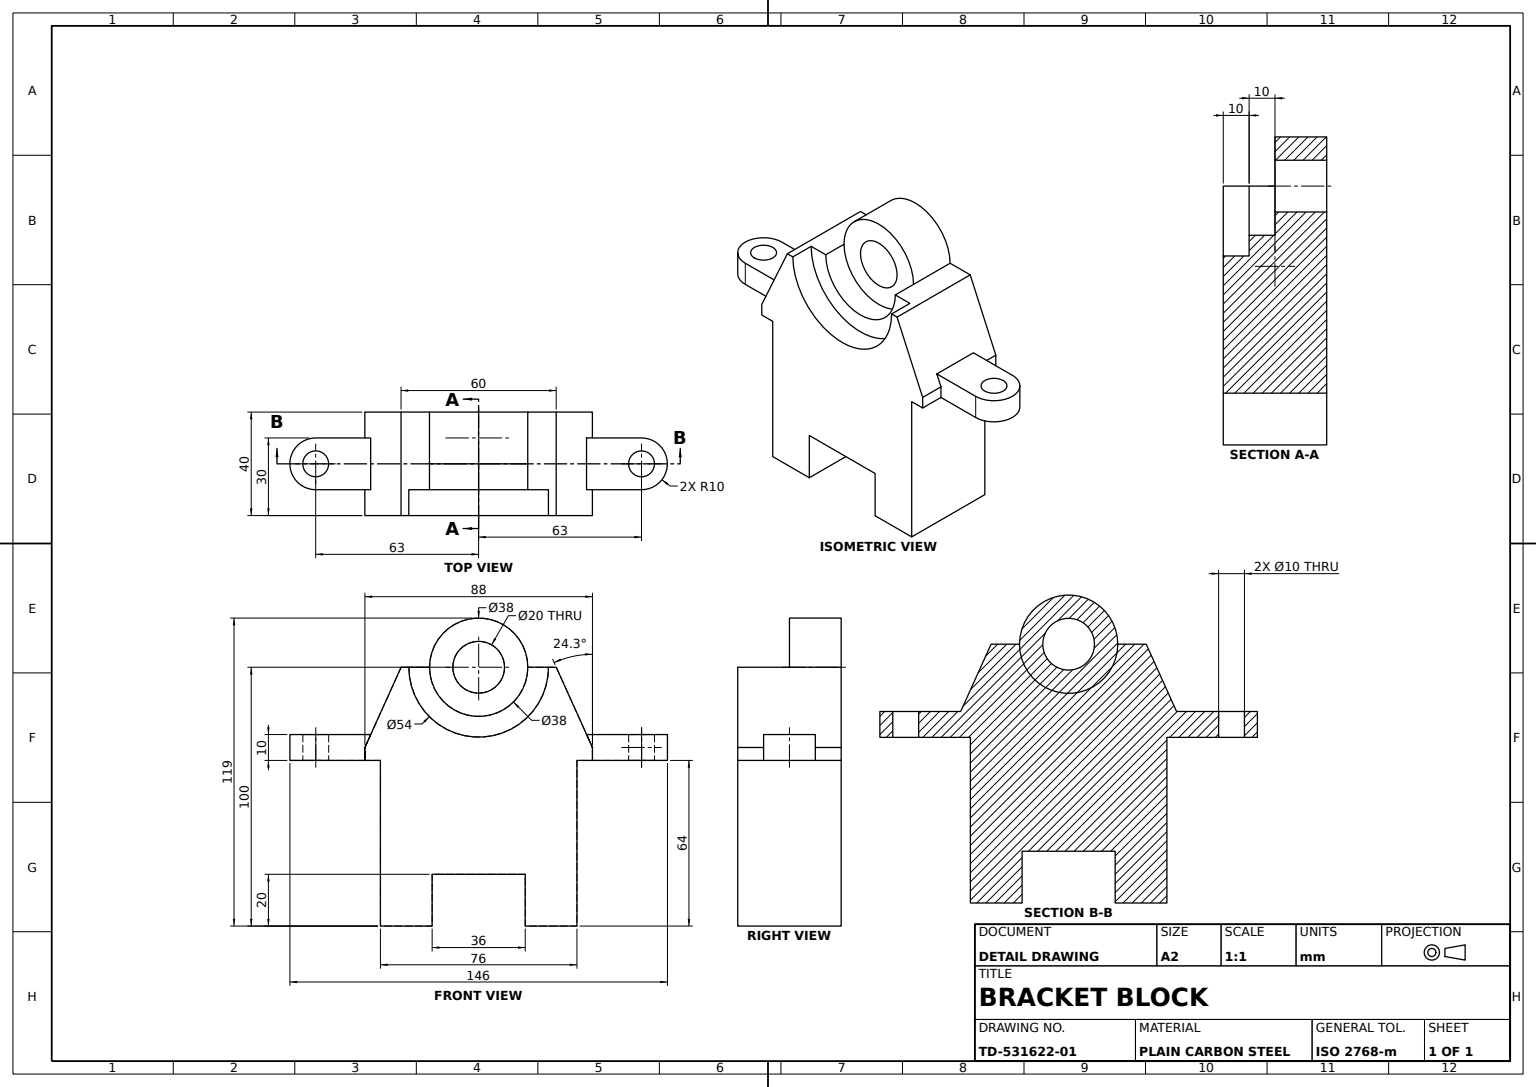
SolidWorks part; units mm, degrees
material "Plain Carbon Steel"
ref_plane "Front Plane" through (0, 0, 0) normal (0, 0, 1) x (1, 0, 0)
ref_plane "Top Plane" through (0, 0, 0) normal (0, 1, 0) x (1, 0, 0)
ref_plane "Right Plane" through (0, 0, 0) normal (1, 0, 0) x (0, 0, -1)
sketch "Pedestal Profile Sketch" plane through (0, 0, 0) normal (0, 0, 1) x (1, 0, 0)
  line L0 (18, -32) -> (38, -32)
  line L1 (-38, -32) -> (-18, -32)
  line L2 (-38, -32) -> (-38, 32)
  line L4 (38, -32) -> (38, 32)
  line L5 (-38, -32) -> (38, 32) construction
  line L6 (-38, 32) -> (38, -32) construction
  line L8 (-18, -32) -> (-18, -12)
  line L9 (-18, -12) -> (18, -12)
  line L10 (18, -32) -> (18, -12)
  line L11 (-38, 32) -> (-44, 32)
  line L12 (-44, 32) -> (-44, 37)
  line L13 (-44, 37) -> (-30, 68)
  line L14 (-30, 68) -> (30, 68)
  line L15 (30, 68) -> (44, 37)
  line L16 (44, 37) -> (44, 32)
  line L17 (44, 32) -> (38, 32)
  line L18 (0, 0) -> (0, 18.857) construction
  point P0 (0, 0)
  point P10 (0, -12)
  point P19 (0, 68)
  dimension "D1" = 76
  dimension "D2" = 36
  dimension "D3" = 20
  dimension "D4" = 36
  dimension "D5" = 64
  dimension "D6" = 5
  dimension "D7" = 88
  dimension "D8" = 60
extrude "Pedestal Body" add sketch "Pedestal Profile Sketch" along normal mid plane 40
sketch "Front Recess Ø54 Sketch" plane through (0, 0, 20) normal (0, 0, 1) x (1, 0, 0)
  line L0 (30, 68) -> (-30, 68) construction
  circle A0 centre (0, 68) radius 27
  dimension "D1" = 54
extrude "Front Recess Ø54" cut sketch "Front Recess Ø54 Sketch" against normal blind 10
sketch "Inner Recess Ø38 Sketch" plane through (0, 0, 10) normal (0, 0, 1) x (1, 0, 0)
  line L0 (27, 68) -> (-27, 68) construction
  circle A0 centre (0, 68) radius 19
  dimension "D1" = 38
extrude "Inner Recess Ø38" cut sketch "Inner Recess Ø38 Sketch" against normal blind 10
sketch "Hub Ø38 Sketch" plane through (0, 0, 0) normal (0, 0, 1) x (1, 0, 0)
  line L0 (19, 68) -> (-19, 68) construction
  circle A0 centre (0, 68) radius 19
  dimension "D1" = 38
extrude "Hub Ø38" add sketch "Hub Ø38 Sketch" against normal up to surface (20 mm away) up to face at (0, 13.2857, -20)
sketch "Bore Ø20 Sketch" plane through (0, 0, 0) normal (0, 0, 1) x (1, 0, 0)
  circle A0 centre (0, 68) radius 10
  dimension "D1" = 20
extrude "Bore Ø20" cut sketch "Bore Ø20 Sketch" against normal through all
sketch "Mounting Ear Sketch" plane through (0, 32, 0) normal (0, -1, 0) x (1, 0, 0)
  line L0 (-44, 0) -> (-63, 0) construction
  line L1 (-44, 20) -> (-44, -20) construction
  line L2 (-63, 10) -> (-44, 10)
  line L3 (-63, -10) -> (-44, -10)
  line L5 (-44, 10) -> (-38, 10)
  line L6 (-38, 20) -> (-38, -20) construction
  line L7 (-38, 10) -> (-38, -10)
  line L8 (-38, 20) -> (-38, -20) construction
  line L9 (-38, -10) -> (-44, -10)
  arc A0 (-63, 10) -> (-63, -10) centre (-63, 0) ccw
  circle A1 centre (-63, 0) radius 5
  dimension "D1" = 10
  dimension "D3" = 10
  dimension "D2" = 63
extrude "Mounting Ear" add sketch "Mounting Ear Sketch" against normal blind 10
mirror "Mounting Ear Mirror" about plane through (0, 0, 0) normal (1, 0, 0) of "Mounting Ear"
